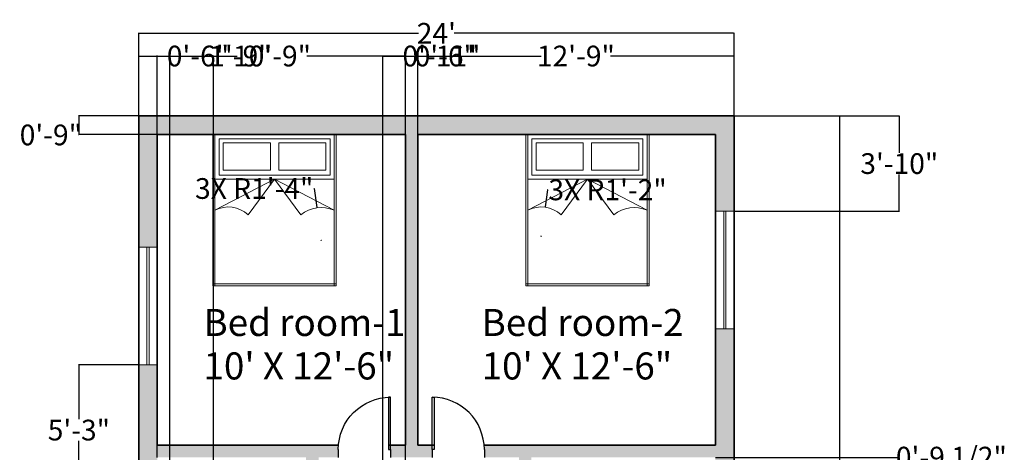
# Model space of a CAD drawing. Units: inches. Extents: x 46 to 946, y 121 to 740.
# Tile 4 of 4: x 57 to 533, y 531 to 740. Entities that reach past the tile are written whole.
import ezdxf

# ---------------------------------------------------------------- set-up
doc = ezdxf.new("R2010")
doc.units = ezdxf.units.IN
doc.header["$MEASUREMENT"] = 0
for name, color, linetype, lineweight in [('A-ANNO-DIMS', 2, 'Continuous', 18), ('A-AREA-IDEN', 7, 'Continuous', 25), ('A-DOOR', 3, 'Continuous', 25), ('A-FURN', 8, 'Continuous', 18), ('A-GLAZ', 4, 'Continuous', 18), ('A-WALL', 7, 'Continuous', 35), ('A-WALL-PATT', 8, 'Continuous', 13)]:
    doc.layers.add(name, color=color, linetype=linetype, lineweight=lineweight)
doc.styles.get("Standard").update_dxf_attribs({"font": 'arial.ttf'})
doc.dimstyles.get("Standard").update_dxf_attribs({"dimtxt": 10, "dimasz": 0.18, "dimexe": 0.18, "dimexo": 0.0625, "dimgap": 0.09, "dimtad": 0, "dimtih": 1, "dimtoh": 1, "dimdec": 0, "dimzin": 0, "dimdsep": 46, "dimlunit": 3, "dimtxsty": 'Standard', "dimcen": 0.09, "dimadec": 0, "dimazin": 0, "dimtfac": 1, "dimtdec": 0, "dimtofl": 0, "dimtmove": 0, "dimatfit": 3, "dimfxl": 1, "dimtolj": 1, "dimtzin": 0, "dimarcsym": 0})

# ---------------------------------------------------------------- blocks, each defined once
blk = doc.blocks.new('*U3')
for p, q in [((0, 0), (0, -6)), ((40, 0), (40, -6))]:
    blk.add_line(p, q)
blk.add_lwpolyline([(0, 0), (0, 40), (1.75, 40), (1.75, 0)], close=True)
blk.add_arc((0, 0), 40, 0, 90)
blk = doc.blocks.new('*D10')
at = {"layer": 'A-ANNO-DIMS', "color": 0, "lineweight": -2, "transparency": 16777216}
for p, q in [((114.48, 693.52), (114.48, 733.57)), ((402.48, 693.52), (402.48, 733.57)), ((114.66, 733.39), (249.82, 733.39)), ((402.3, 733.39), (267.14, 733.39))]:
    blk.add_line(p, q, dxfattribs=at)
at = {"layer": 'A-ANNO-DIMS', "color": 0, "transparency": 16777216}
for points in [[(114.66, 733.42), (114.66, 733.36), (114.48, 733.39)], [(402.3, 733.42), (402.3, 733.36), (402.48, 733.39)]]:
    blk.add_solid(points, dxfattribs=at)
at = {"layer": 'Defpoints', "color": 0, "transparency": 16777216}
for p in [(402.48, 733.39), (114.48, 693.46), (402.48, 693.46)]:
    blk.add_point(p, dxfattribs=at)
at = {"layer": 'A-ANNO-DIMS', "color": 0, "transparency": 16777216, "insert": (258.48, 733.39), "char_height": 10, "attachment_point": 5}
blk.add_mtext("\\A1;24'", dxfattribs=at)
blk = doc.blocks.new('*D11')
at = {"layer": 'A-ANNO-DIMS', "color": 0, "lineweight": -2, "transparency": 16777216}
for p, q in [((402.54, 693.46), (453.64, 693.46)), ((453.46, 693.28), (453.46, 446.07)), ((453.46, 188.64), (453.46, 435.85)), ((402.54, 188.46), (453.64, 188.46))]:
    blk.add_line(p, q, dxfattribs=at)
at = {"layer": 'A-ANNO-DIMS', "color": 0, "transparency": 16777216}
for points in [[(453.43, 693.28), (453.49, 693.28), (453.46, 693.46)], [(453.43, 188.64), (453.49, 188.64), (453.46, 188.46)]]:
    blk.add_solid(points, dxfattribs=at)
at = {"layer": 'Defpoints', "color": 0, "transparency": 16777216}
for p in [(402.48, 693.46), (402.48, 188.46), (453.46, 188.46)]:
    blk.add_point(p, dxfattribs=at)
at = {"layer": 'A-ANNO-DIMS', "color": 0, "transparency": 16777216, "insert": (453.46, 440.96), "char_height": 10, "attachment_point": 5}
blk.add_mtext('\\A1;42\'-1"', dxfattribs=at)
blk = doc.blocks.new('WIN-56_82IN')
for p, q in [((9, 56.82), (0, 56.82)), ((0, 0), (0, 56.82)), ((4, 56.82), (4, 0)), ((5, 56.82), (5, 0)), ((9, 56.82), (9, 0)), ((9, 0), (0, 0))]:
    blk.add_line(p, q)
blk = doc.blocks.new('BED-DOUBLE')
for p, q in [((0, 73.15), (0, 0)), ((1, 73.15), (1, 0)), ((58.72, 0), (58.72, 73.15)), ((59.72, 0), (59.72, 73.15)), ((29.86, 51.59), (1, 36.57)), ((29.86, 51.59), (17.08, 34.42)), ((29.86, 51.59), (58.72, 36.57)), ((29.86, 51.59), (42.63, 34.42)), ((0, 1), (59.72, 1)), ((0, 0), (59.72, 0))]:
    blk.add_line(p, q)
for points in [[(1, 73.15), (58.72, 73.15), (58.72, 51.59), (1, 51.59)], [(3, 71.15), (56.72, 71.15), (56.72, 53.59), (3, 53.59)], [(5, 69.15), (27.85, 69.15), (27.85, 55.92), (5, 55.92)], [(54.72, 69.15), (31.87, 69.15), (31.87, 55.92), (54.72, 55.92)]]:
    blk.add_lwpolyline(points, close=True)
for centre, radius, start, end in [((7.51, 24.06), 14.1, 47.2425, 117.4957), ((52.47, 22.1), 15.76, 66.6553, 128.6065)]:
    blk.add_arc(centre, radius, start, end)
blk = doc.blocks.new('*D19')
at = {"layer": 'A-ANNO-DIMS', "color": 0, "lineweight": -2, "transparency": 16777216}
for p, q in [((114.48, 510.3), (114.48, 518.94)), ((114.66, 518.76), (123.3, 518.76)), ((123.48, 510.3), (123.48, 518.94)), ((123.48, 518.76), (123.66, 518.76))]:
    blk.add_line(p, q, dxfattribs=at)
at = {"layer": 'A-ANNO-DIMS', "color": 0, "transparency": 16777216}
for points in [[(114.66, 518.79), (114.66, 518.73), (114.48, 518.76)], [(123.3, 518.79), (123.3, 518.73), (123.48, 518.76)]]:
    blk.add_solid(points, dxfattribs=at)
at = {"layer": 'Defpoints', "color": 0, "transparency": 16777216}
for p in [(123.48, 518.76), (114.48, 510.24), (123.48, 510.24)]:
    blk.add_point(p, dxfattribs=at)
at = {"layer": 'A-ANNO-DIMS', "color": 0, "transparency": 16777216, "insert": (154.22, 518.76), "char_height": 10, "attachment_point": 5}
blk.add_mtext('\\A1;0\'-9" TYP.', dxfattribs=at)
blk = doc.blocks.new('*D27')
at = {"layer": 'A-ANNO-DIMS', "color": 0, "lineweight": -2, "transparency": 16777216}
for p, q in [((114.41, 693.46), (85.35, 693.46)), ((85.53, 693.28), (85.53, 684.64)), ((123.41, 684.46), (85.35, 684.46)), ((85.53, 684.28), (85.35, 684.28)), ((85.53, 684.46), (85.53, 684.28))]:
    blk.add_line(p, q, dxfattribs=at)
at = {"layer": 'A-ANNO-DIMS', "color": 0, "transparency": 16777216}
for points in [[(85.5, 693.28), (85.56, 693.28), (85.53, 693.46)], [(85.5, 684.64), (85.56, 684.64), (85.53, 684.46)]]:
    blk.add_solid(points, dxfattribs=at)
at = {"layer": 'Defpoints', "color": 0, "transparency": 16777216}
for p in [(114.48, 693.46), (85.53, 684.46), (123.48, 684.46)]:
    blk.add_point(p, dxfattribs=at)
at = {"layer": 'A-ANNO-DIMS', "color": 0, "transparency": 16777216, "insert": (71.97, 684.28), "char_height": 10, "attachment_point": 5}
blk.add_mtext('\\A1;0\'-9"', dxfattribs=at)
blk = doc.blocks.new('*D28')
at = {"layer": 'A-ANNO-DIMS', "color": 0, "lineweight": -2, "transparency": 16777216}
for p, q in [((114.48, 693.52), (114.48, 722.59)), ((114.66, 722.41), (162.18, 722.41)), ((243.3, 722.41), (195.77, 722.41)), ((243.48, 684.52), (243.48, 722.59))]:
    blk.add_line(p, q, dxfattribs=at)
at = {"layer": 'A-ANNO-DIMS', "color": 0, "transparency": 16777216}
for points in [[(114.66, 722.44), (114.66, 722.38), (114.48, 722.41)], [(243.3, 722.44), (243.3, 722.38), (243.48, 722.41)]]:
    blk.add_solid(points, dxfattribs=at)
at = {"layer": 'Defpoints', "color": 0, "transparency": 16777216}
for p in [(243.48, 722.41), (114.48, 693.46), (243.48, 684.46)]:
    blk.add_point(p, dxfattribs=at)
at = {"layer": 'A-ANNO-DIMS', "color": 0, "transparency": 16777216, "insert": (178.98, 722.41), "char_height": 10, "attachment_point": 5}
blk.add_mtext('\\A1;10\'-9"', dxfattribs=at)
blk = doc.blocks.new('*D29')
at = {"layer": 'A-ANNO-DIMS', "color": 0, "lineweight": -2, "transparency": 16777216}
for p, q in [((243.48, 684.52), (243.48, 722.59)), ((243.66, 722.41), (249.3, 722.41)), ((249.48, 684.52), (249.48, 722.59)), ((249.48, 722.41), (249.66, 722.41))]:
    blk.add_line(p, q, dxfattribs=at)
at = {"layer": 'A-ANNO-DIMS', "color": 0, "transparency": 16777216}
for points in [[(243.66, 722.44), (243.66, 722.38), (243.48, 722.41)], [(249.3, 722.44), (249.3, 722.38), (249.48, 722.41)]]:
    blk.add_solid(points, dxfattribs=at)
at = {"layer": 'Defpoints', "color": 0, "transparency": 16777216}
for p in [(249.48, 722.41), (243.48, 684.46), (249.48, 684.46)]:
    blk.add_point(p, dxfattribs=at)
at = {"layer": 'A-ANNO-DIMS', "color": 0, "transparency": 16777216, "insert": (263.04, 722.41), "char_height": 10, "attachment_point": 5}
blk.add_mtext('\\A1;0\'-6"', dxfattribs=at)
blk = doc.blocks.new('*D30')
at = {"layer": 'A-ANNO-DIMS', "color": 0, "lineweight": -2, "transparency": 16777216}
for p, q in [((249.48, 684.52), (249.48, 722.59)), ((249.66, 722.41), (309.18, 722.41)), ((402.3, 722.41), (342.77, 722.41)), ((402.48, 693.52), (402.48, 722.59))]:
    blk.add_line(p, q, dxfattribs=at)
at = {"layer": 'A-ANNO-DIMS', "color": 0, "transparency": 16777216}
for points in [[(249.66, 722.44), (249.66, 722.38), (249.48, 722.41)], [(402.3, 722.44), (402.3, 722.38), (402.48, 722.41)]]:
    blk.add_solid(points, dxfattribs=at)
at = {"layer": 'Defpoints', "color": 0, "transparency": 16777216}
for p in [(402.48, 722.41), (402.48, 693.46), (249.48, 684.46)]:
    blk.add_point(p, dxfattribs=at)
at = {"layer": 'A-ANNO-DIMS', "color": 0, "transparency": 16777216, "insert": (325.98, 722.41), "char_height": 10, "attachment_point": 5}
blk.add_mtext('\\A1;12\'-9"', dxfattribs=at)
blk = doc.blocks.new('*D36')
at = {"layer": 'A-ANNO-DIMS', "color": 0, "lineweight": -2, "transparency": 16777216}
for p, q in [((114.41, 573.18), (85.35, 573.18)), ((85.53, 573), (85.53, 546.91)), ((85.53, 510.42), (85.53, 536.51)), ((114.41, 510.24), (85.35, 510.24))]:
    blk.add_line(p, q, dxfattribs=at)
at = {"layer": 'A-ANNO-DIMS', "color": 0, "transparency": 16777216}
for points in [[(85.5, 573), (85.56, 573), (85.53, 573.18)], [(85.5, 510.42), (85.56, 510.42), (85.53, 510.24)]]:
    blk.add_solid(points, dxfattribs=at)
at = {"layer": 'Defpoints', "color": 0, "transparency": 16777216}
for p in [(85.53, 573.18), (114.48, 573.18), (114.48, 510.24)]:
    blk.add_point(p, dxfattribs=at)
at = {"layer": 'A-ANNO-DIMS', "color": 0, "transparency": 16777216, "insert": (85.53, 541.71), "char_height": 10, "attachment_point": 5}
blk.add_mtext('\\A1;5\'-3"', dxfattribs=at)
blk = doc.blocks.new('*D40')
at = {"layer": 'A-ANNO-DIMS', "color": 0, "lineweight": -2, "transparency": 16777216}
for p, q in [((393.54, 528.46), (482.61, 528.46)), ((482.43, 528.46), (482.43, 528.64)), ((482.43, 528.64), (482.61, 528.64)), ((482.43, 519.05), (482.43, 528.28)), ((402.54, 518.87), (482.61, 518.87))]:
    blk.add_line(p, q, dxfattribs=at)
at = {"layer": 'A-ANNO-DIMS', "color": 0, "transparency": 16777216}
for points in [[(482.4, 528.28), (482.46, 528.28), (482.43, 528.46)], [(482.4, 519.05), (482.46, 519.05), (482.43, 518.87)]]:
    blk.add_solid(points, dxfattribs=at)
at = {"layer": 'Defpoints', "color": 0, "transparency": 16777216}
for p in [(393.48, 528.46), (482.43, 528.46), (402.48, 518.87)]:
    blk.add_point(p, dxfattribs=at)
at = {"layer": 'A-ANNO-DIMS', "color": 0, "transparency": 16777216, "insert": (507.64, 528.64), "char_height": 10, "attachment_point": 5}
blk.add_mtext('\\A1;0\'-9 1/2"', dxfattribs=at)
blk = doc.blocks.new('*D42')
at = {"layer": 'A-ANNO-DIMS', "color": 0, "lineweight": -2, "transparency": 16777216}
for p, q in [((402.54, 693.46), (482.61, 693.46)), ((482.43, 693.28), (482.43, 675.64)), ((482.43, 647.6), (482.43, 665.24)), ((402.54, 647.42), (482.61, 647.42))]:
    blk.add_line(p, q, dxfattribs=at)
at = {"layer": 'A-ANNO-DIMS', "color": 0, "transparency": 16777216}
for points in [[(482.4, 693.28), (482.46, 693.28), (482.43, 693.46)], [(482.4, 647.6), (482.46, 647.6), (482.43, 647.42)]]:
    blk.add_solid(points, dxfattribs=at)
at = {"layer": 'Defpoints', "color": 0, "transparency": 16777216}
for p in [(402.48, 693.46), (482.43, 693.46), (402.48, 647.42)]:
    blk.add_point(p, dxfattribs=at)
at = {"layer": 'A-ANNO-DIMS', "color": 0, "transparency": 16777216, "insert": (482.43, 670.44), "char_height": 10, "attachment_point": 5}
blk.add_mtext('\\A1;3\'-10"', dxfattribs=at)
blk = doc.blocks.new('*D45')
at = {"layer": 'A-ANNO-DIMS', "color": 0, "lineweight": -2, "transparency": 16777216}
for p, q in [((129.58, 470.61), (129.58, 722.59)), ((129.76, 722.41), (150.42, 722.41)), ((150.6, 470.61), (150.6, 722.59)), ((150.6, 722.41), (150.78, 722.41))]:
    blk.add_line(p, q, dxfattribs=at)
at = {"layer": 'A-ANNO-DIMS', "color": 0, "transparency": 16777216}
for points in [[(129.76, 722.44), (129.76, 722.38), (129.58, 722.41)], [(150.42, 722.44), (150.42, 722.38), (150.6, 722.41)]]:
    blk.add_solid(points, dxfattribs=at)
at = {"layer": 'Defpoints', "color": 0, "transparency": 16777216}
for p in [(150.6, 722.41), (129.58, 470.54), (150.6, 470.54)]:
    blk.add_point(p, dxfattribs=at)
at = {"layer": 'A-ANNO-DIMS', "color": 0, "transparency": 16777216, "insert": (163.69, 722.41), "char_height": 10, "attachment_point": 5}
blk.add_mtext('\\A1;1\'-9"', dxfattribs=at)
blk = doc.blocks.new('*D65')
at = {"layer": 'A-ANNO-DIMS', "color": 0, "lineweight": -2, "transparency": 16777216}
for p, q in [((232.61, 426.52), (232.61, 722.59)), ((232.79, 722.41), (243.3, 722.41)), ((243.48, 426.52), (243.48, 722.59)), ((243.48, 722.41), (243.66, 722.41))]:
    blk.add_line(p, q, dxfattribs=at)
at = {"layer": 'A-ANNO-DIMS', "color": 0, "transparency": 16777216}
for points in [[(232.79, 722.44), (232.79, 722.38), (232.61, 722.41)], [(243.3, 722.44), (243.3, 722.38), (243.48, 722.41)]]:
    blk.add_solid(points, dxfattribs=at)
at = {"layer": 'Defpoints', "color": 0, "transparency": 16777216}
for p in [(243.48, 722.41), (232.61, 426.46), (243.48, 426.46)]:
    blk.add_point(p, dxfattribs=at)
at = {"layer": 'A-ANNO-DIMS', "color": 0, "transparency": 16777216, "insert": (260.92, 722.41), "char_height": 10, "attachment_point": 5}
blk.add_mtext('\\A1;0\'-11"', dxfattribs=at)
blk = doc.blocks.new('*D66')
at = {"layer": 'A-ANNO-DIMS', "color": 0, "lineweight": -2, "transparency": 16777216}
for p, q in [((123.48, 528.52), (123.48, 722.59)), ((123.66, 722.41), (129.4, 722.41)), ((129.58, 513.74), (129.58, 722.59)), ((129.58, 722.41), (129.76, 722.41))]:
    blk.add_line(p, q, dxfattribs=at)
at = {"layer": 'A-ANNO-DIMS', "color": 0, "transparency": 16777216}
for points in [[(123.66, 722.44), (123.66, 722.38), (123.48, 722.41)], [(129.4, 722.44), (129.4, 722.38), (129.58, 722.41)]]:
    blk.add_solid(points, dxfattribs=at)
at = {"layer": 'Defpoints', "color": 0, "transparency": 16777216}
for p in [(129.58, 722.41), (123.48, 528.46), (129.58, 513.68)]:
    blk.add_point(p, dxfattribs=at)
at = {"layer": 'A-ANNO-DIMS', "color": 0, "transparency": 16777216, "insert": (143.14, 722.41), "char_height": 10, "attachment_point": 5}
blk.add_mtext('\\A1;0\'-6"', dxfattribs=at)
blk = doc.blocks.new('*D73')
at = {"layer": 'A-ANNO-DIMS', "color": 0, "lineweight": -2, "transparency": 16777216}
for p, q in [((199.26, 658.41), (199.44, 658.41)), ((199.44, 658.41), (200.67, 649.22)), ((202.7, 633.41), (202.88, 633.41)), ((202.79, 633.32), (202.79, 633.5))]:
    blk.add_line(p, q, dxfattribs=at)
at = {"layer": 'A-ANNO-DIMS', "color": 0, "transparency": 16777216}
blk.add_solid([(200.7, 649.22), (200.64, 649.21), (200.69, 649.04)], dxfattribs=at)
at = {"layer": 'Defpoints', "color": 0, "transparency": 16777216}
for p in [(200.69, 649.04), (202.79, 633.41)]:
    blk.add_point(p, dxfattribs=at)
at = {"layer": 'A-ANNO-DIMS', "color": 0, "transparency": 16777216, "insert": (170.35, 658.41), "char_height": 10, "attachment_point": 5}
blk.add_mtext('\\A1;3X R1\'-4"', dxfattribs=at)
blk = doc.blocks.new('*D74')
at = {"layer": 'A-ANNO-DIMS', "color": 0, "lineweight": -2, "transparency": 16777216}
for p, q in [((312.21, 657.74), (311.11, 649.54)), ((312.39, 657.74), (312.21, 657.74)), ((309.13, 635.38), (309.31, 635.38)), ((309.22, 635.29), (309.22, 635.47))]:
    blk.add_line(p, q, dxfattribs=at)
at = {"layer": 'A-ANNO-DIMS', "color": 0, "transparency": 16777216}
blk.add_solid([(311.09, 649.54), (311.14, 649.53), (311.09, 649.36)], dxfattribs=at)
at = {"layer": 'Defpoints', "color": 0, "transparency": 16777216}
for p in [(311.09, 649.36), (309.22, 635.38)]:
    blk.add_point(p, dxfattribs=at)
at = {"layer": 'A-ANNO-DIMS', "color": 0, "transparency": 16777216, "insert": (341.3, 657.74), "char_height": 10, "attachment_point": 5}
blk.add_mtext('\\A1;3X R1\'-2"', dxfattribs=at)

msp = doc.modelspace()

# ---------------------------------------------------------------- hatches: boundary and pattern name
at = {"layer": 'A-WALL-PATT'}
h = msp.add_hatch(color=256, dxfattribs=at)
h.dxf.hatch_style = 1
h.paths.add_polyline_path([(256.37, 197.46), (249.48, 197.46), (249.48, 258.28), (245.68, 258.28, -0.021769), (243.48, 258.37), (243.48, 197.46), (221.61, 197.46), (221.61, 188.46), (243.48, 188.46), (256.37, 188.46), (256.37, 192.26)])
h.paths.add_polyline_path([(164.78, 197.46), (123.48, 197.46), (123.48, 224.01), (114.48, 224.01), (114.48, 188.46), (164.78, 188.46)])
h.paths.add_polyline_path([(402.48, 216.63), (393.48, 216.63), (393.48, 197.46), (327.48, 197.46), (281.15, 197.46, -0.051771), (281.69, 192.26), (281.69, 188.46), (402.48, 188.46)])
h.paths.add_polyline_path([(123.48, 346.49), (114.48, 346.49), (114.48, 280.83), (123.48, 280.83), (123.48, 299.46), (243.48, 299.46), (243.48, 283.6), (245.68, 283.6), (249.48, 283.6), (249.48, 299.46), (256.37, 299.46), (256.37, 303.26), (256.37, 304.46), (249.48, 304.46), (249.48, 432.46), (243.48, 432.46), (232.61, 432.46), (232.61, 426.46), (243.48, 426.46), (243.48, 305.46), (123.48, 305.46)])
h.paths.add_polyline_path([(231.5, 428.66), (232.61, 428.66), (232.61, 403.34), (231.5, 403.34), (231.5, 403.37, -0.376395), (207.38, 426.46), (123.48, 426.46), (123.48, 403.31), (114.48, 403.31), (114.48, 453.42), (123.48, 453.42), (123.48, 432.46), (195.48, 432.46), (195.48, 474.9), (201.48, 474.9), (201.48, 432.46), (207.29, 432.46), (207.29, 428.66, 0.401453), (231.5, 403.37)])
h.paths.add_polyline_path([(211.14, 534.46), (123.48, 534.46), (123.48, 573.18), (114.48, 573.18), (114.48, 510.24), (123.48, 510.24), (123.48, 528.46), (195.48, 528.46), (195.48, 495.84), (201.48, 495.84), (201.48, 528.46), (211.04, 528.46), (211.04, 532.26, -0.021769)])
h.paths.add_polyline_path([(123.48, 684.46), (243.48, 684.46), (243.48, 534.46), (236.36, 534.46), (236.36, 532.26), (236.36, 528.46), (256.37, 528.46), (256.37, 532.26), (256.37, 534.46), (249.48, 534.46), (249.48, 684.46), (393.48, 684.46), (393.48, 647.42), (402.48, 647.42), (402.48, 693.46), (114.48, 693.46), (114.48, 630), (123.48, 630)])
h.paths.add_polyline_path([(402.48, 590.59), (393.48, 590.59), (393.48, 534.46), (281.59, 534.46, -0.021769), (281.69, 532.26), (281.69, 528.46), (298.48, 528.46), (298.48, 518.41), (302.28, 518.41), (304.48, 518.41), (304.48, 528.46), (393.48, 528.46), (393.48, 518.87), (402.48, 518.87)])
h.paths.add_polyline_path([(402.48, 500.87), (393.48, 500.87), (393.48, 482.46), (304.48, 482.46), (304.48, 493.19, -0.021769), (302.28, 493.09), (298.48, 493.09), (298.48, 482.46), (298.48, 476.46), (304.48, 476.46), (393.48, 476.46), (393.48, 455.17), (402.48, 455.17)])
h.paths.add_polyline_path([(402.48, 419.17), (393.48, 419.17), (393.48, 356.8), (402.48, 356.8)])
h.paths.add_polyline_path([(358.48, 304.46), (281.66, 304.46, -0.01187), (281.69, 303.26), (281.69, 299.46), (358.48, 299.46)])

# ---------------------------------------------------------------- linework, layer by layer
at = {"layer": 'A-FURN'}
for p, q in [((151.32, 684.46), (209.03, 684.46)), ((209.03, 684.46), (209.03, 684.46)), ((209.03, 684.46), (209.03, 680.78))]:
    msp.add_line(p, q, dxfattribs=at)
at = {"layer": 'A-WALL'}
for p, q in [((114.48, 693.46), (114.48, 188.46)), ((114.48, 693.46), (402.48, 693.46)), ((114.48, 693.46), (402.48, 693.46)), ((402.48, 693.46), (402.48, 693.46)), ((402.48, 693.46), (402.48, 188.46)), ((123.48, 684.46), (123.48, 534.46)), ((123.48, 684.46), (243.48, 684.46)), ((243.48, 684.46), (243.48, 534.46)), ((249.48, 684.46), (249.48, 534.46)), ((249.48, 684.46), (393.48, 684.46)), ((393.48, 684.46), (393.48, 534.46)), ((123.48, 534.46), (211.14, 534.46)), ((235.26, 534.46), (243.48, 534.46)), ((249.48, 534.46), (257.48, 534.46)), ((281.59, 534.46), (393.48, 534.46))]:
    msp.add_line(p, q, dxfattribs=at)

# ---------------------------------------------------------------- block references
at = {"layer": 'A-DOOR', "yscale": 0.6330408260540115, "zscale": 0.6330408260540115}
for p, xscale in [((236.36, 532.26), -0.6330408260540115), ((256.37, 532.26), 0.6330408260540115)]:
    msp.add_blockref('*U3', p, dxfattribs=dict(at, xscale=xscale))
at = {"layer": 'A-FURN'}
for p in [(150.32, 611.32), (301.71, 611.32)]:
    msp.add_blockref('BED-DOUBLE', p, dxfattribs=at)
at = {"layer": 'A-GLAZ'}
for p in [(393.48, 590.59), (114.48, 573.18)]:
    msp.add_blockref('WIN-56_82IN', p, dxfattribs=at)

# ---------------------------------------------------------------- texts
at = {"layer": 'A-AREA-IDEN'}
for s, height, p in [('Bed room-1', 13.067, (145.81, 587.15)), ('Bed room-2', 13.067, (280.37, 587.15)), ('10\' X 12\'-6"', 13.0671, (145.81, 566.16)), ('10\' X 12\'-6"', 13.0671, (280.37, 566.16))]:
    msp.add_text(s, height=height, dxfattribs=at).set_placement(p)

# ---------------------------------------------------------------- dimensions: what is measured, and where the dimension line sits
at = {"layer": 'A-ANNO-DIMS'}
for base, p1, p2, override, picture, middle in [((402.48, 733.39), (114.48, 693.46), (402.48, 693.46), {"dimclrd": 0, "dimclre": 0, "dimclrt": 0}, '*D10', (258.48, 733.39)), ((243.48, 722.41), (114.48, 693.46), (243.48, 684.46), {"dimdec": 1, "dimlfac": 1, "dimrnd": 0, "dimzin": 1, "dimdsep": 46, "dimlunit": 4, "dimfrac": 2}, '*D28', (178.98, 722.41)), ((129.58, 722.41), (123.48, 528.46), (129.58, 513.68), {"dimdec": 1, "dimlfac": 1, "dimrnd": 0, "dimzin": 1, "dimdsep": 46, "dimlunit": 4, "dimfrac": 2}, '*D66', (143.14, 722.41)), ((150.6, 722.41), (129.58, 470.54), (150.6, 470.54), {"dimdec": 1, "dimlfac": 1, "dimrnd": 0, "dimzin": 1, "dimdsep": 46, "dimlunit": 4, "dimfrac": 2}, '*D45', (163.69, 722.41)), ((243.48, 722.41), (232.61, 426.46), (243.48, 426.46), {"dimdec": 1, "dimlfac": 1, "dimrnd": 0, "dimzin": 1, "dimdsep": 46, "dimlunit": 4, "dimfrac": 2}, '*D65', (260.92, 722.41)), ((249.48, 722.41), (243.48, 684.46), (249.48, 684.46), {"dimdec": 1, "dimlfac": 1, "dimrnd": 0, "dimzin": 1, "dimdsep": 46, "dimlunit": 4, "dimfrac": 2}, '*D29', (263.04, 722.41)), ((402.48, 722.41), (249.48, 684.46), (402.48, 693.46), {"dimdec": 1, "dimlfac": 1, "dimrnd": 0, "dimzin": 1, "dimdsep": 46, "dimlunit": 4, "dimfrac": 2}, '*D30', (325.98, 722.41))]:
    dim = msp.add_linear_dim(base=base, p1=p1, p2=p2, dimstyle='Standard', override=override, dxfattribs=at)
    dim.commit()
    dim.dimension.update_dxf_attribs({"geometry": picture, "text_midpoint": middle})
for base, p1, p2, override, picture, middle in [((85.53, 684.46), (114.48, 693.46), (123.48, 684.46), {"dimdec": 1, "dimlfac": 1, "dimrnd": 0, "dimzin": 1, "dimdsep": 46, "dimlunit": 4, "dimfrac": 2}, '*D27', (71.97, 684.28)), ((453.46, 188.46), (402.48, 693.46), (402.48, 188.46), {"dimclrd": 0, "dimclre": 0, "dimclrt": 0}, '*D11', (453.46, 440.96)), ((482.43, 693.46), (402.48, 647.42), (402.48, 693.46), {"dimdec": 1, "dimlfac": 1, "dimrnd": 0, "dimzin": 1, "dimdsep": 46, "dimlunit": 4, "dimfrac": 2}, '*D42', (482.43, 670.44)), ((85.53, 573.18), (114.48, 510.24), (114.48, 573.18), {"dimdec": 1, "dimlfac": 1, "dimrnd": 0, "dimzin": 1, "dimdsep": 46, "dimlunit": 4, "dimfrac": 2}, '*D36', (85.53, 541.71)), ((482.43, 528.46), (402.48, 518.87), (393.48, 528.46), {"dimdec": 1, "dimlfac": 1, "dimrnd": 0, "dimzin": 1, "dimdsep": 46, "dimlunit": 4, "dimfrac": 2}, '*D40', (507.64, 528.64))]:
    dim = msp.add_linear_dim(base=base, p1=p1, p2=p2, angle=90, dimstyle='Standard', override=override, dxfattribs=at)
    dim.commit()
    dim.dimension.update_dxf_attribs({"geometry": picture, "text_midpoint": middle})
for center, mpoint, picture, middle in [((202.79, 633.41), (200.69, 649.04), '*D73', (170.35, 658.41)), ((309.22, 635.38), (311.09, 649.36), '*D74', (341.3, 657.74))]:
    dim = msp.add_radius_dim(center=center, mpoint=mpoint, text='3X <>', dimstyle='Standard', override={"dimdec": 1, "dimlfac": 1, "dimrnd": 0, "dimzin": 1, "dimdsep": 46, "dimlunit": 4, "dimfrac": 2}, dxfattribs=at)
    dim.commit()
    dim.dimension.update_dxf_attribs({"geometry": picture, "text_midpoint": middle, "dimtype": 164})
dim = msp.add_linear_dim(base=(123.48, 518.76), p1=(114.48, 510.24), p2=(123.48, 510.24), text='<> TYP.', dimstyle='Standard', override={"dimdec": 1, "dimlfac": 1, "dimrnd": 0, "dimzin": 1, "dimdsep": 46, "dimlunit": 4, "dimfrac": 2}, dxfattribs=at)
dim.commit()
dim.dimension.update_dxf_attribs({"geometry": '*D19', "text_midpoint": (154.22, 518.76)})

doc.saveas('drawing.dxf')
